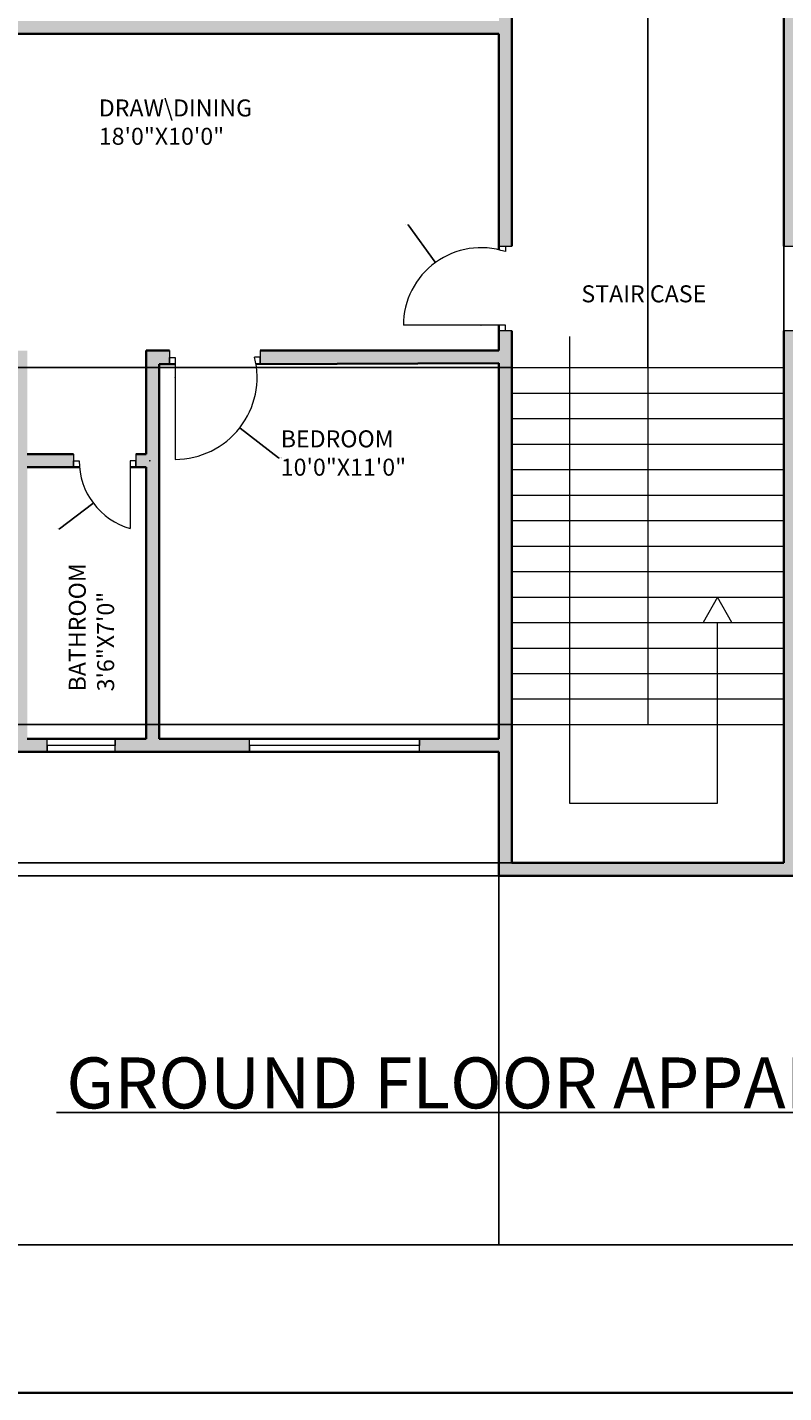
# Model space of a CAD drawing. Units: inches. Extents: x 2314 to 3223, y 1382 to 2735.
# Tile 2 of 14: x 2551 to 2818, y 1382 to 1864. Entities that reach past the tile are written whole.
import ezdxf

# ---------------------------------------------------------------- set-up
doc = ezdxf.new("R2010")
doc.units = ezdxf.units.IN
for name, color, linetype, lineweight in [('A-ANNO-DIMS', 2, 'Continuous', 18), ('A-ANNO-TEXT', 7, 'Continuous', 25), ('A-ANNO-TTLB', 7, 'Continuous', 35), ('A-AREA-IDEN', 7, 'Continuous', 18), ('A-DOOR', 3, 'Continuous', 18), ('A-FLOR-STRS', 7, 'Continuous', 18), ('A-GLAZ', 4, 'Continuous', 18), ('A-WALL', 7, 'Continuous', 35)]:
    doc.layers.add(name, color=color, linetype=linetype, lineweight=lineweight)
doc.layers.add('A-WALL-PATT', color=251, linetype='Continuous', lineweight=13, true_color=0x636466)
doc.styles.get("Standard").update_dxf_attribs({"font": 'arial.ttf'})
doc.dimstyles.get("Standard").update_dxf_attribs({"dimtxt": 0.18, "dimasz": 0.18, "dimexe": 0.18, "dimexo": 0.0625, "dimgap": 0.09, "dimtad": 0, "dimtih": 1, "dimtoh": 1, "dimdec": 4, "dimzin": 0, "dimdsep": 46, "dimtxsty": 'Standard', "dimcen": 0.09, "dimadec": 0, "dimazin": 0, "dimtfac": 1, "dimtdec": 4, "dimtofl": 0, "dimtmove": 0, "dimatfit": 3, "dimfxl": 1, "dimtolj": 1, "dimtzin": 0, "dimarcsym": 0})

# ---------------------------------------------------------------- blocks, each defined once
blk = doc.blocks.new('WIN-PLAN-24')
for p, q in [((0, 24), (4.5, 24)), ((4.5, 24), (2.25, 24)), ((2.25, 24), (2.25, 0)), ((2.25, 0), (0, 0)), ((0, 0), (4.5, 0))]:
    blk.add_line(p, q)
blk = doc.blocks.new('WIN-PLAN-60')
for p, q in [((0, 4.5), (0, 0)), ((0, 0), (0, 2.25)), ((0, 2.25), (60, 2.25)), ((60, 2.25), (60, 4.5)), ((60, 4.5), (60, 0))]:
    blk.add_line(p, q)
blk = doc.blocks.new('*D29')
at = {"layer": 'A-ANNO-DIMS', "color": 0, "lineweight": -2, "transparency": 16777216}
for p, q in [((2410.39, 1608.32), (2410.39, 1434.13)), ((3125.89, 1608.32), (3125.89, 1434.13)), ((2410.57, 1434.31), (2767.75, 1434.31)), ((3125.71, 1434.31), (2768.54, 1434.31))]:
    blk.add_line(p, q, dxfattribs=at)
at = {"layer": 'A-ANNO-DIMS', "color": 0, "transparency": 16777216}
for points in [[(2410.57, 1434.34), (2410.57, 1434.28), (2410.39, 1434.31)], [(3125.71, 1434.34), (3125.71, 1434.28), (3125.89, 1434.31)]]:
    blk.add_solid(points, dxfattribs=at)
at = {"layer": 'Defpoints', "color": 0, "transparency": 16777216}
for p in [(2410.39, 1608.38), (3125.89, 1608.38), (3125.89, 1434.31)]:
    blk.add_point(p, dxfattribs=at)
at = {"layer": 'A-ANNO-DIMS', "color": 0, "transparency": 16777216, "insert": (2768.14, 1434.31), "char_height": 0.18, "attachment_point": 5}
blk.add_mtext('\\A1;715.5', dxfattribs=at)
blk = doc.blocks.new('*D31')
at = {"layer": 'A-ANNO-DIMS', "color": 0, "lineweight": -2, "transparency": 16777216}
for p, q in [((2410.33, 1608.38), (2363.51, 1608.38)), ((2363.69, 1608.2), (2363.69, 1586.68)), ((2363.69, 1564.8), (2363.69, 1586.32)), ((2717.83, 1564.62), (2363.51, 1564.62))]:
    blk.add_line(p, q, dxfattribs=at)
at = {"layer": 'A-ANNO-DIMS', "color": 0, "transparency": 16777216}
for points in [[(2363.66, 1608.2), (2363.72, 1608.2), (2363.69, 1608.38)], [(2363.66, 1564.8), (2363.72, 1564.8), (2363.69, 1564.62)]]:
    blk.add_solid(points, dxfattribs=at)
at = {"layer": 'Defpoints', "color": 0, "transparency": 16777216}
for p in [(2363.69, 1608.38), (2410.39, 1608.38), (2717.89, 1564.62)]:
    blk.add_point(p, dxfattribs=at)
at = {"layer": 'A-ANNO-DIMS', "color": 0, "transparency": 16777216, "insert": (2363.69, 1586.5), "char_height": 0.18, "attachment_point": 5}
blk.add_mtext('\\A1;43.76', dxfattribs=at)
blk = doc.blocks.new('*D35')
at = {"layer": 'A-ANNO-DIMS', "color": 0, "lineweight": -2, "transparency": 16777216}
for p, q in [((2722.33, 1744), (2363.51, 1744)), ((2363.69, 1743.82), (2363.69, 1681.18)), ((2363.69, 1618.18), (2363.69, 1680.82)), ((2722.33, 1618), (2363.51, 1618))]:
    blk.add_line(p, q, dxfattribs=at)
at = {"layer": 'A-ANNO-DIMS', "color": 0, "transparency": 16777216}
for points in [[(2363.66, 1743.82), (2363.72, 1743.82), (2363.69, 1744)], [(2363.66, 1618.18), (2363.72, 1618.18), (2363.69, 1618)]]:
    blk.add_solid(points, dxfattribs=at)
at = {"layer": 'Defpoints', "color": 0, "transparency": 16777216}
for p in [(2363.69, 1744), (2722.39, 1744), (2722.39, 1618)]:
    blk.add_point(p, dxfattribs=at)
at = {"layer": 'A-ANNO-DIMS', "color": 0, "transparency": 16777216, "insert": (2363.69, 1681), "char_height": 0.18, "attachment_point": 5}
blk.add_mtext('\\A1;126', dxfattribs=at)
blk = doc.blocks.new('*D36')
at = {"layer": 'A-ANNO-DIMS', "color": 0, "lineweight": -2, "transparency": 16777216}
for p, q in [((2722.33, 1618), (2363.51, 1618)), ((2363.69, 1617.82), (2363.69, 1593.74)), ((2363.69, 1569.3), (2363.69, 1593.38)), ((2722.33, 1569.12), (2363.51, 1569.12))]:
    blk.add_line(p, q, dxfattribs=at)
at = {"layer": 'A-ANNO-DIMS', "color": 0, "transparency": 16777216}
for points in [[(2363.66, 1617.82), (2363.72, 1617.82), (2363.69, 1618)], [(2363.66, 1569.3), (2363.72, 1569.3), (2363.69, 1569.12)]]:
    blk.add_solid(points, dxfattribs=at)
at = {"layer": 'Defpoints', "color": 0, "transparency": 16777216}
for p in [(2363.69, 1618), (2722.39, 1618), (2722.39, 1569.12)]:
    blk.add_point(p, dxfattribs=at)
at = {"layer": 'A-ANNO-DIMS', "color": 0, "transparency": 16777216, "insert": (2363.69, 1593.56), "char_height": 0.18, "attachment_point": 5}
blk.add_mtext('\\A1;48.88', dxfattribs=at)
blk = doc.blocks.new('*D37')
at = {"layer": 'A-ANNO-DIMS', "color": 0, "lineweight": -2, "transparency": 16777216}
for p, q in [((2717.89, 1564.56), (2717.89, 1434.13)), ((2822.89, 1564.56), (2822.89, 1434.13)), ((2718.07, 1434.31), (2770.11, 1434.31)), ((2822.71, 1434.31), (2770.67, 1434.31))]:
    blk.add_line(p, q, dxfattribs=at)
at = {"layer": 'A-ANNO-DIMS', "color": 0, "transparency": 16777216}
for points in [[(2718.07, 1434.34), (2718.07, 1434.28), (2717.89, 1434.31)], [(2822.71, 1434.34), (2822.71, 1434.28), (2822.89, 1434.31)]]:
    blk.add_solid(points, dxfattribs=at)
at = {"layer": 'Defpoints', "color": 0, "transparency": 16777216}
for p in [(2717.89, 1564.62), (2822.89, 1564.62), (2822.89, 1434.31)]:
    blk.add_point(p, dxfattribs=at)
at = {"layer": 'A-ANNO-DIMS', "color": 0, "transparency": 16777216, "insert": (2770.39, 1434.31), "char_height": 0.18, "attachment_point": 5}
blk.add_mtext('\\A1;105', dxfattribs=at)
blk = doc.blocks.new('*D39')
at = {"layer": 'A-ANNO-DIMS', "color": 0, "lineweight": -2, "transparency": 16777216}
for p, q in [((2770.39, 1744.06), (2770.39, 2428.66)), ((2770.57, 2428.48), (2794.17, 2428.48)), ((2818.21, 2428.48), (2794.62, 2428.48)), ((2818.39, 1744.06), (2818.39, 2428.66))]:
    blk.add_line(p, q, dxfattribs=at)
at = {"layer": 'A-ANNO-DIMS', "color": 0, "transparency": 16777216}
for points in [[(2770.57, 2428.51), (2770.57, 2428.45), (2770.39, 2428.48)], [(2818.21, 2428.51), (2818.21, 2428.45), (2818.39, 2428.48)]]:
    blk.add_solid(points, dxfattribs=at)
at = {"layer": 'Defpoints', "color": 0, "transparency": 16777216}
for p in [(2818.39, 2428.48), (2770.39, 1744), (2818.39, 1744)]:
    blk.add_point(p, dxfattribs=at)
at = {"layer": 'A-ANNO-DIMS', "color": 0, "transparency": 16777216, "insert": (2794.39, 2428.48), "char_height": 0.18, "attachment_point": 5}
blk.add_mtext('\\A1;48', dxfattribs=at)
blk = doc.blocks.new('*D71')
at = {"layer": 'A-ANNO-DIMS', "color": 0, "lineweight": -2, "transparency": 16777216}
for p, q in [((2603.49, 1740.53), (2603.67, 1740.53)), ((2603.58, 1740.44), (2603.58, 1740.62)), ((2640.12, 1712.09), (2626.56, 1722.65)), ((2640.3, 1712.09), (2640.12, 1712.09))]:
    blk.add_line(p, q, dxfattribs=at)
at = {"layer": 'A-ANNO-DIMS', "color": 0, "transparency": 16777216}
blk.add_solid([(2626.58, 1722.67), (2626.54, 1722.62), (2626.42, 1722.76)], dxfattribs=at)
at = {"layer": 'Defpoints', "color": 0, "transparency": 16777216}
for p in [(2603.58, 1740.53), (2626.42, 1722.76)]:
    blk.add_point(p, dxfattribs=at)
at = {"layer": 'A-ANNO-DIMS', "color": 0, "transparency": 16777216, "insert": (2640.78, 1712.09), "char_height": 0.18, "attachment_point": 5}
blk.add_mtext('\\A1;R28.94', dxfattribs=at)
blk = doc.blocks.new('*D76')
at = {"layer": 'A-ANNO-DIMS', "color": 0, "lineweight": -2, "transparency": 16777216}
for p, q in [((2685.69, 1794.45), (2685.87, 1794.45)), ((2685.87, 1794.45), (2695.39, 1781.27)), ((2711.45, 1758.92), (2711.63, 1758.92)), ((2711.54, 1758.83), (2711.54, 1759.01))]:
    blk.add_line(p, q, dxfattribs=at)
at = {"layer": 'A-ANNO-DIMS', "color": 0, "transparency": 16777216}
blk.add_solid([(2695.41, 1781.29), (2695.37, 1781.25), (2695.5, 1781.12)], dxfattribs=at)
at = {"layer": 'Defpoints', "color": 0, "transparency": 16777216}
for p in [(2695.5, 1781.12), (2711.54, 1758.92)]:
    blk.add_point(p, dxfattribs=at)
at = {"layer": 'A-ANNO-DIMS', "color": 0, "transparency": 16777216, "insert": (2685.14, 1794.45), "char_height": 0.18, "attachment_point": 5}
blk.add_mtext('\\A1;R27.393', dxfattribs=at)
blk = doc.blocks.new('*D81')
at = {"layer": 'A-ANNO-DIMS', "color": 0, "lineweight": -2, "transparency": 16777216}
for p, q in [((2594.56, 1711.13), (2594.74, 1711.13)), ((2594.65, 1711.04), (2594.65, 1711.22)), ((2562.74, 1687.09), (2574.56, 1696)), ((2562.56, 1687.09), (2562.74, 1687.09))]:
    blk.add_line(p, q, dxfattribs=at)
at = {"layer": 'A-ANNO-DIMS', "color": 0, "transparency": 16777216}
blk.add_solid([(2574.54, 1696.02), (2574.58, 1695.98), (2574.7, 1696.11)], dxfattribs=at)
at = {"layer": 'Defpoints', "color": 0, "transparency": 16777216}
for p in [(2594.65, 1711.13), (2574.7, 1696.11)]:
    blk.add_point(p, dxfattribs=at)
at = {"layer": 'A-ANNO-DIMS', "color": 0, "transparency": 16777216, "insert": (2562.08, 1687.09), "char_height": 0.18, "attachment_point": 5}
blk.add_mtext('\\A1;R24.97', dxfattribs=at)

msp = doc.modelspace()

# ---------------------------------------------------------------- hatches: boundary and pattern name
at = {"layer": 'A-WALL-PATT'}
h = msp.add_hatch(color=256, dxfattribs=at)
h.dxf.hatch_style = 1
h.paths.add_polyline_path([(2443.3302, 2379.5332), (2443.3302, 2381.7832), (2410.3927, 2381.7832), (2410.3927, 2336.7008), (2414.8927, 2336.7008), (2414.8927, 2377.2832), (2443.3302, 2377.2832)])
h.paths.add_polyline_path([(2561.3645, 2379.5332), (2561.3645, 2381.7832), (2503.3302, 2381.7832), (2503.3302, 2377.2832), (2546.8927, 2377.2832), (2546.8927, 2245.2832), (2541.8787, 2245.2832), (2541.8787, 2240.7832), (2551.3927, 2240.7832), (2551.3927, 2377.2832), (2561.3645, 2377.2832)])
h.paths.add_polyline_path([(2656.0607, 2381.7832), (2597.3645, 2381.7832), (2597.3645, 2377.2832), (2617.3927, 2377.2832), (2617.3927, 2257.2832), (2584.2532, 2257.2832), (2584.2532, 2252.7832), (2625.8528, 2252.7832), (2625.8528, 2255.0332), (2625.8528, 2257.2832), (2621.8927, 2257.2832), (2621.8927, 2377.2832), (2656.0607, 2377.2832), (2656.0607, 2379.5332)])
h.paths.add_polyline_path([(2807.3418, 2381.7832), (2716.0607, 2381.7832), (2716.0607, 2377.2832), (2765.8927, 2377.2832), (2765.8927, 2257.2832), (2661.6935, 2257.2832), (2661.6935, 2252.7832), (2765.8927, 2252.7832), (2765.8927, 2146.2832), (2760.9259, 2146.2832), (2760.9259, 2141.8832), (2775.7119, 2141.8832), (2775.7119, 2146.2832), (2770.3927, 2146.2832), (2770.3927, 2252.7832), (2877.684, 2252.7832), (2877.684, 2255.0332), (2877.684, 2257.2832), (2770.3927, 2257.2832), (2770.3927, 2377.2832), (2807.3418, 2377.2832), (2807.3418, 2379.5332)])
h.paths.add_polyline_path([(2937.2118, 2381.7832), (2867.3418, 2381.7832), (2867.3418, 2377.2832), (2914.3927, 2377.2832), (2914.3927, 2257.2832), (2908.4124, 2257.2832), (2908.4124, 2252.7832), (2960.6432, 2252.7832), (2960.6432, 2255.0332), (2960.6432, 2257.2832), (2918.8927, 2257.2832), (2918.8927, 2377.2832), (2937.2118, 2377.2832)])
h.paths.add_polyline_path([(3022.1601, 2381.7832), (2973.2118, 2381.7832), (2973.2118, 2379.5332), (2973.2118, 2377.2832), (2984.8927, 2377.2832), (2984.8927, 2257.2832), (2980.0601, 2257.2832), (2980.0601, 2252.7832), (2984.8927, 2252.7832), (2984.8927, 2240.7832), (2995.668, 2240.7832), (2995.668, 2243.0332), (2995.668, 2245.2832), (2989.3927, 2245.2832), (2989.3927, 2377.2832), (3022.1601, 2377.2832), (3022.1601, 2379.5332)])
h.paths.add_polyline_path([(3125.8927, 2381.7832), (3082.1601, 2381.7832), (3082.1601, 2377.2832), (3121.3927, 2377.2832), (3121.3927, 2334.7388), (3125.8927, 2334.7388)])
h.paths.add_polyline_path([(3125.8927, 2274.7388), (3121.3927, 2274.7388), (3121.3927, 2245.2832), (3066.4832, 2245.2832), (3066.4832, 2240.7832), (3121.3927, 2240.7832), (3121.3927, 2232.1868), (3125.8927, 2232.1868)])
h.paths.add_polyline_path([(3125.8927, 2208.1868), (3121.3927, 2208.1868), (3121.3927, 2198.7832), (3037.3927, 2198.7832), (3037.3927, 2240.7832), (3041.2694, 2240.7832), (3041.2694, 2243.0332), (3041.2694, 2245.2832), (3026.8205, 2245.2832), (3026.8205, 2240.7832), (3032.8927, 2240.7832), (3032.8927, 2190.4022), (3037.3927, 2190.4022), (3037.3927, 2194.2832), (3121.3927, 2194.2832), (3121.3927, 2182.1835), (3125.8927, 2182.1835)])
h.paths.add_polyline_path([(3125.8927, 2158.1835), (3121.3927, 2158.1835), (3121.3927, 2146.2832), (3037.3927, 2146.2832), (3037.3927, 2169.3726), (3035.1427, 2169.3726), (3032.8927, 2169.3726), (3032.8927, 2146.2832), (2812.7301, 2146.2832), (2812.7301, 2144.0832), (2812.7301, 2141.8832), (2818.3927, 2141.8832), (2818.3927, 1970.1316), (2822.8927, 1970.1316), (2822.8927, 1978.8832), (2903.9846, 1978.8832), (2903.9846, 1981.1332), (2903.9846, 1983.3832), (2822.8927, 1983.3832), (2822.8927, 2115.3832), (2851.7162, 2115.3832), (2851.7162, 2117.6332), (2851.7162, 2119.8832), (2822.8927, 2119.8832), (2822.8927, 2141.8832), (3125.8927, 2141.8832)])
h.paths.add_polyline_path([(3125.8927, 2119.8832), (3081.193, 2119.8832), (3081.193, 2115.3832), (3121.3927, 2115.3832), (3121.3927, 2071.8188), (3125.8927, 2071.8188)], flags=17)
h.paths.add_polyline_path([(2989.3927, 2115.3832), (3021.193, 2115.3832), (3021.193, 2117.6332), (3021.193, 2119.8832), (2979.123, 2119.8832), (2979.123, 2115.3832), (2984.8927, 2115.3832), (2984.8927, 2019.3832), (2981.9225, 2019.3832), (2981.9225, 2014.8832), (2984.8927, 2014.8832), (2984.8927, 1983.3832), (2984.8927, 1978.8832), (2989.3927, 1978.8832), (2989.3927, 1983.3832)], flags=17)
h.paths.add_polyline_path([(2947.3927, 2115.3832), (2955.123, 2115.3832), (2955.123, 2117.6332), (2955.123, 2119.8832), (2911.7162, 2119.8832), (2911.7162, 2115.3832), (2942.8927, 2115.3832), (2942.8927, 1983.3832), (2936.7017, 1983.3832), (2936.7017, 1978.8832), (2947.3927, 1978.8832), (2947.3927, 1983.3832), (2947.3927, 2014.8832), (2960.7167, 2014.8832), (2960.7167, 2017.1332), (2960.7167, 2019.3832), (2947.3927, 2019.3832)], flags=17)
h.paths.add_polyline_path([(3037.3927, 1978.8832), (3041.8276, 1978.8832), (3041.8276, 1981.1332), (3041.8276, 1983.3832), (3025.477, 1983.3832), (3025.477, 1978.8832), (3032.8927, 1978.8832), (3032.8927, 1927.1259), (3035.1427, 1927.1259), (3037.3927, 1927.1259)])
h.paths.add_polyline_path([(3125.8927, 2011.8188), (3123.6427, 2011.8188), (3121.3927, 2011.8188), (3121.3927, 1983.3832), (3065, 1983.3832), (3065, 1978.8832), (3121.3927, 1978.8832), (3121.3927, 1970.5932), (3125.8927, 1970.5932)], flags=17)
h.paths.add_polyline_path([(2994.2341, 1983.3832), (2989.3927, 1983.3832), (2989.3927, 1978.8832), (2994.2341, 1978.8832), (2994.2341, 1981.1332)], flags=16)
h.paths.add_polyline_path([(3125.8927, 1946.5932), (3121.3927, 1946.5932), (3121.3927, 1936.8832), (3037.3927, 1936.8832), (3037.3927, 1932.3832), (3121.3927, 1932.3832), (3121.3927, 1919.825), (3125.8927, 1919.825)])
h.paths.add_polyline_path([(3125.8927, 1883.825), (3121.3927, 1883.825), (3121.3927, 1866.3832), (3037.3927, 1866.3832), (3037.3927, 1899.0954), (3035.1427, 1899.0954), (3032.8927, 1899.0954), (3032.8927, 1866.3832), (2822.8927, 1866.3832), (2822.8927, 1938.7212), (2820.6427, 1938.7212), (2818.3927, 1938.7212), (2818.3927, 1786.9239), (2822.8927, 1786.9239), (2822.8927, 1861.8832), (3032.8927, 1861.8832), (3032.8927, 1825.1023), (3037.3927, 1825.1023), (3037.3927, 1861.8832), (3121.3927, 1861.8832), (3121.3927, 1844.6765), (3125.8927, 1844.6765)])
h.paths.add_polyline_path([(3125.8927, 1808.6765), (3121.3927, 1808.6765), (3121.3927, 1795.8832), (3037.3927, 1795.8832), (3037.3927, 1799.4755), (3032.8927, 1799.4755), (3032.8927, 1749.3832), (3026.5034, 1749.3832), (3026.5034, 1744.8832), (3032.8927, 1744.8832), (3034.9255, 1744.8832), (3043.1326, 1744.8832), (3043.1326, 1747.1332), (3043.1326, 1749.3832), (3037.3927, 1749.3832), (3037.3927, 1791.3832), (3121.3927, 1791.3832), (3121.3927, 1783.3103), (3125.8927, 1783.3103)])
h.paths.add_polyline_path([(3125.8927, 1759.3103), (3121.3927, 1759.3103), (3121.3927, 1749.3832), (3065.1845, 1749.3832), (3065.1845, 1744.8832), (3121.3927, 1744.8832), (3121.3927, 1709.3573), (3125.8927, 1709.3573)])
h.paths.add_polyline_path([(3125.8927, 1649.3573), (3121.3927, 1649.3573), (3121.3927, 1612.8832), (3095.116, 1612.8832), (3095.116, 1608.3832), (3125.8927, 1608.3832)])
h.paths.add_polyline_path([(3035.116, 1612.8832), (2993.8927, 1612.8832), (2993.8927, 1744.8832), (2998.7409, 1744.8832), (2998.7409, 1749.3832), (2989.3927, 1749.3832), (2989.3927, 1744.8832), (2989.3927, 1701.3832), (2972.8226, 1701.3832), (2972.8226, 1696.8832), (2989.3927, 1696.8832), (2989.3927, 1612.8832), (2978.2225, 1612.8832), (2978.2225, 1608.3832), (3035.116, 1608.3832), (3035.116, 1610.6332)])
h.paths.add_polyline_path([(2947.3927, 1696.8832), (2950.7566, 1696.8832), (2950.7566, 1699.1332), (2950.7566, 1701.3832), (2947.3927, 1701.3832), (2947.3927, 1744.8832), (2947.3927, 1749.3832), (2937.649, 1749.3832), (2937.649, 1744.8832), (2942.8927, 1744.8832), (2942.8927, 1612.8832), (2907.783, 1612.8832), (2907.783, 1608.3832), (2954.2225, 1608.3832), (2954.2225, 1610.6332), (2954.2225, 1612.8832), (2947.3927, 1612.8832)])
h.paths.add_polyline_path([(2822.8927, 1744.8832), (2905.3491, 1744.8832), (2905.3491, 1747.1332), (2905.3491, 1749.3832), (2822.8927, 1749.3832), (2822.8927, 1756.9185), (2818.3927, 1756.9185), (2818.3927, 1612.8832), (2818.3927, 1569.1205), (2722.3927, 1569.1205), (2722.3927, 1612.8832), (2722.3927, 1756.9185), (2717.8927, 1756.9185), (2717.8927, 1750.0143), (2633.6297, 1750.0143), (2633.6437, 1745.2665), (2717.8927, 1745.5143), (2717.8927, 1612.8832), (2689.8467, 1612.8832), (2689.8467, 1608.3832), (2717.8927, 1608.3832), (2717.8927, 1564.6205), (2722.3927, 1564.6205), (2822.8927, 1564.6205), (2822.8927, 1569.1205), (2822.8927, 1608.3832), (2847.783, 1608.3832), (2847.783, 1610.6332), (2847.783, 1612.8832), (2822.8927, 1612.8832)])
h.paths.add_polyline_path([(2629.8467, 1612.8832), (2597.8927, 1612.8832), (2597.8927, 1744.8832), (2597.8927, 1745.1613), (2601.5887, 1745.1721), (2601.5816, 1747.5932), (2601.5745, 1750.0143), (2593.3927, 1750.0143), (2593.3927, 1744.8832), (2593.3927, 1713.3832), (2589.7588, 1713.3832), (2589.7588, 1708.8832), (2593.3927, 1708.8832), (2593.3927, 1612.8832), (2582.3793, 1612.8832), (2582.3793, 1608.3832), (2629.8467, 1608.3832), (2629.8467, 1610.6332)])
h.paths.add_polyline_path([(2551.3927, 1708.8832), (2567.6776, 1708.8832), (2567.6776, 1711.1332), (2567.6776, 1713.3832), (2551.3927, 1713.3832), (2551.3927, 1744.8832), (2551.3927, 1750.0143), (2543.5657, 1750.0143), (2543.5657, 1747.5079), (2543.5657, 1745.0014), (2546.8927, 1745.0112), (2546.8927, 1744.8832), (2546.8927, 1612.8832), (2502.9339, 1612.8832), (2502.9339, 1608.3832), (2558.3793, 1608.3832), (2558.3793, 1610.6332), (2558.3793, 1612.8832), (2551.3927, 1612.8832)])
h.paths.add_polyline_path([(2414.8927, 1656.2547), (2410.3927, 1656.2547), (2410.3927, 1608.3832), (2442.9339, 1608.3832), (2442.9339, 1610.6332), (2442.9339, 1612.8832), (2414.8927, 1612.8832)])
h.paths.add_polyline_path([(2414.8927, 1744.8832), (2468.8906, 1744.8832), (2468.8906, 1747.1332), (2468.8906, 1749.3832), (2414.8927, 1749.3832), (2414.8927, 1757.7622), (2410.3927, 1757.7622), (2410.3927, 1716.2547), (2414.8927, 1716.2547)])
h.paths.add_polyline_path([(2414.8927, 1791.3832), (2498.8927, 1791.3832), (2498.8927, 1749.3832), (2492.9799, 1749.3832), (2492.9799, 1744.8832), (2498.8927, 1744.8832), (2503.3927, 1744.8832), (2508.0135, 1744.8968), (2508.0059, 1747.4556), (2507.9984, 1750.0143), (2503.3927, 1750.0143), (2503.3927, 1802.6362), (2501.1427, 1802.6362), (2498.8927, 1802.6362), (2498.8927, 1795.8832), (2414.8927, 1795.8832), (2414.8927, 1808.0943), (2410.3927, 1808.0943), (2410.3927, 1781.7622), (2414.8927, 1781.7622)])
h.paths.add_polyline_path([(2722.3927, 1937.589), (2720.1427, 1937.589), (2717.8927, 1937.589), (2717.8927, 1866.3832), (2503.3927, 1866.3832), (2503.3927, 1896.3484), (2498.8927, 1896.3484), (2498.8927, 1866.3832), (2414.8927, 1866.3832), (2414.8927, 1882.1496), (2410.3927, 1882.1496), (2410.3927, 1844.0943), (2414.8927, 1844.0943), (2414.8927, 1861.8832), (2498.8927, 1861.8832), (2498.8927, 1831.4783), (2501.1427, 1831.4783), (2503.3927, 1831.4783), (2503.3927, 1861.8832), (2717.8927, 1861.8832), (2717.8927, 1786.9239), (2722.3927, 1786.9239)])
h.paths.add_polyline_path([(2414.8927, 1932.3832), (2498.8927, 1932.3832), (2498.8927, 1924.7883), (2503.3927, 1924.7883), (2503.3927, 1978.8832), (2505.8599, 1978.8832), (2505.8599, 1981.1332), (2505.8599, 1983.3832), (2493.3697, 1983.3832), (2493.3697, 1978.8832), (2498.8927, 1978.8832), (2498.8927, 1936.8832), (2414.8927, 1936.8832), (2414.8927, 1943.2834), (2410.3927, 1943.2834), (2410.3927, 1918.1496), (2414.8927, 1918.1496)])
h.paths.add_polyline_path([(2414.8927, 2020.3133), (2412.6427, 2020.3133), (2410.3927, 2020.3133), (2410.3927, 1967.2834), (2414.8927, 1967.2834), (2414.8927, 1978.8832), (2468.8513, 1978.8832), (2468.8513, 1981.1332), (2468.8513, 1983.3832), (2414.8927, 1983.3832)])
h.paths.add_polyline_path([(2414.8927, 2115.3832), (2453.004, 2115.3832), (2453.004, 2117.6332), (2453.004, 2119.8832), (2410.3927, 2119.8832), (2410.3927, 2080.3133), (2414.8927, 2080.3133)], flags=17)
h.paths.add_polyline_path([(2559.0969, 2117.6332), (2559.0969, 2119.8832), (2513.004, 2119.8832), (2513.004, 2115.3832), (2546.8927, 2115.3832), (2546.8927, 1983.3832), (2542.7531, 1983.3832), (2542.7531, 1978.8832), (2551.3927, 1978.8832), (2551.3927, 2014.8832), (2570.3098, 2014.8832), (2570.3098, 2017.1332), (2570.3098, 2019.3832), (2551.3927, 2019.3832), (2551.3927, 2115.3832), (2559.0969, 2115.3832)], flags=17)
h.paths.add_polyline_path([(2628.5073, 2117.6332), (2628.5073, 2119.8832), (2583.0969, 2119.8832), (2583.0969, 2115.3832), (2593.3927, 2115.3832), (2593.3927, 2019.3832), (2590.2108, 2019.3832), (2590.2108, 2014.8832), (2593.3927, 2014.8832), (2593.3927, 1978.8832), (2601.5907, 1978.8832), (2601.5907, 1981.1332), (2601.5907, 1983.3832), (2597.8927, 1983.3832), (2597.8927, 2115.3832), (2628.5073, 2115.3832)], flags=17)
h.paths.add_polyline_path([(2722.3927, 2141.8832), (2726.9871, 2141.8832), (2726.9871, 2144.2705), (2726.9871, 2146.2832), (2503.3927, 2146.2832), (2503.3927, 2168.2161), (2501.1427, 2168.2161), (2498.8927, 2168.2161), (2498.8927, 2146.2832), (2414.8927, 2146.2832), (2414.8927, 2156.5041), (2410.3927, 2156.5041), (2410.3927, 2141.8832), (2717.8927, 2141.8832), (2717.8927, 2119.8832), (2688.5073, 2119.8832), (2688.5073, 2115.3832), (2717.8927, 2115.3832), (2717.8927, 1983.3832), (2633.2454, 1983.3832), (2633.2454, 1978.8832), (2717.8927, 1978.8832), (2717.8927, 1970.1316), (2720.1427, 1970.1316), (2722.3927, 1970.1316)])
h.paths.add_polyline_path([(2557.3704, 1462.9278), (2940.0934, 1462.9278), (2940.0934, 1512.3848), (2557.3704, 1512.3848)], flags=9)
h.paths.add_polyline_path([(2846.2527, 1703.1384), (2892.8612, 1703.1384), (2892.8612, 1725.5272), (2846.2527, 1725.5272)], flags=25)
h.paths.add_polyline_path([(2885.6102, 1812.1147), (2946.1505, 1812.1147), (2946.1505, 1834.5035), (2885.6102, 1834.5035)], flags=25)
h.paths.add_polyline_path([(2885.6102, 1884.183), (2946.1505, 1884.183), (2946.1505, 1906.5718), (2885.6102, 1906.5718)], flags=25)
h.paths.add_polyline_path([(3066.365, 1705.5431), (3112.9735, 1705.5431), (3112.9735, 1727.9319), (3066.365, 1727.9319)], flags=9)
h.paths.add_polyline_path([(3061.8255, 1887.7513), (3101.6154, 1887.7513), (3101.6154, 1910.1401), (3061.8255, 1910.1401)], flags=25)
h.paths.add_polyline_path([(3063.3679, 1816.2121), (3103.1578, 1816.2121), (3103.1578, 1838.6009), (3063.3679, 1838.6009)], flags=25)
h.paths.add_polyline_path([(3053.3743, 1768.416), (3107.1329, 1768.416), (3107.1329, 1790.8048), (3053.3743, 1790.8048)], flags=25)
h.paths.add_polyline_path([(3061.6068, 1943.822), (3115.3653, 1943.822), (3115.3653, 1966.2109), (3061.6068, 1966.2109)], flags=9)
h.paths.add_polyline_path([(2745.0978, 1763.6604), (2797.9354, 1763.6604), (2797.9354, 1776.0247), (2745.0978, 1776.0247)], flags=9)
h.paths.add_polyline_path([(2574.2135, 1819.2586), (2634.7538, 1819.2586), (2634.7538, 1841.6474), (2574.2135, 1841.6474)], flags=25)
h.paths.add_polyline_path([(2574.2135, 1891.3269), (2634.7538, 1891.3269), (2634.7538, 1913.7157), (2574.2135, 1913.7157)], flags=25)
h.paths.add_polyline_path([(2638.4466, 1702.43), (2685.0551, 1702.43), (2685.0551, 1724.8188), (2638.4466, 1724.8188)], flags=25)
h.paths.add_polyline_path([(2435.9715, 1697.1215), (2482.5799, 1697.1215), (2482.5799, 1719.5103), (2435.9715, 1719.5103)], flags=9)
h.paths.add_polyline_path([(2431.2046, 1893.7833), (2470.9945, 1893.7833), (2470.9945, 1916.1721), (2431.2046, 1916.1721)], flags=25)
h.paths.add_polyline_path([(2439.8144, 1817.2116), (2479.6043, 1817.2116), (2479.6043, 1839.6004), (2439.8144, 1839.6004)], flags=25)
h.paths.add_polyline_path([(2441.2607, 1753.0942), (2495.0192, 1753.0942), (2495.0192, 1775.483), (2441.2607, 1775.483)], flags=25)
h.paths.add_polyline_path([(2421.216, 1945.3109), (2474.9746, 1945.3109), (2474.9746, 1967.6997), (2421.216, 1967.6997)], flags=25)
h.paths.add_polyline_path([(2585.4464, 1627.5703), (2585.4464, 1679), (2563.0576, 1679), (2563.0576, 1627.5703)], flags=9)
h.paths.add_polyline_path([(2978.3497, 1618.7039), (2978.3497, 1670.1337), (2955.9609, 1670.1337), (2955.9609, 1618.7039)], flags=9)
h.paths.add_polyline_path([(2975.9502, 2041.7828), (2975.9502, 2093.2125), (2953.5614, 2093.2125), (2953.5614, 2041.7828)], flags=25)
h.paths.add_polyline_path([(2835.6537, 1989.2068), (2882.2621, 1989.2068), (2882.2621, 2011.5956), (2835.6537, 2011.5956)], flags=25)
h.paths.add_polyline_path([(2649.3769, 1997.5659), (2695.9853, 1997.5659), (2695.9853, 2019.9547), (2649.3769, 2019.9547)], flags=25)
h.paths.add_polyline_path([(2579.9087, 2040.3429), (2579.9087, 2091.7726), (2557.5198, 2091.7726), (2557.5198, 2040.3429)], flags=25)
h.paths.add_polyline_path([(2783.2404, 1883.1956), (2783.2404, 2067.1369), (2764.694, 2067.1369), (2764.694, 1883.1956)], flags=9)
h.paths.add_polyline_path([(3055.8435, 1993.5571), (3102.4519, 1993.5571), (3102.4519, 2015.9459), (3055.8435, 2015.9459)], flags=25)
h.paths.add_polyline_path([(2423.6009, 1984.6082), (2470.2094, 1984.6082), (2470.2094, 2006.997), (2423.6009, 2006.997)], flags=25)
h.paths.add_polyline_path([(2973.4115, 2123.1668), (3013.1319, 2123.1668), (3013.1319, 2135.531), (2973.4115, 2135.531)], flags=25)
h.paths.add_polyline_path([(2534.3846, 2124.6231), (2574.105, 2124.6231), (2574.105, 2136.9874), (2534.3846, 2136.9874)], flags=25)
h.paths.add_polyline_path([(2829.1368, 2188.1931), (2889.411, 2188.1931), (2889.411, 2210.5819), (2829.1368, 2210.5819)], flags=9)
h.paths.add_polyline_path([(2633.2547, 2185.0437), (2693.5289, 2185.0437), (2693.5289, 2207.4325), (2633.2547, 2207.4325)], flags=9)
h.paths.add_polyline_path([(2445.1812, 2167.0395), (2496.611, 2167.0395), (2496.611, 2189.4284), (2445.1812, 2189.4284)], flags=9)
h.paths.add_polyline_path([(2429.1678, 2194.5482), (2480.5975, 2194.5482), (2480.5975, 2216.937), (2429.1678, 2216.937)], flags=9)
h.paths.add_polyline_path([(3060.1138, 2158.1056), (3111.5436, 2158.1056), (3111.5436, 2180.4944), (3060.1138, 2180.4944)], flags=9)
h.paths.add_polyline_path([(3055.6824, 2201.2631), (3107.1122, 2201.2631), (3107.1122, 2223.652), (3055.6824, 2223.652)], flags=25)
h.paths.add_polyline_path([(3044.3482, 2257.7345), (3090.9567, 2257.7345), (3090.9567, 2280.1233), (3044.3482, 2280.1233)], flags=9)
h.paths.add_polyline_path([(2942.5437, 2306.9625), (2982.3336, 2306.9625), (2982.3336, 2329.3513), (2942.5437, 2329.3513)], flags=9)
h.paths.add_polyline_path([(2799.5865, 2259.1663), (2846.195, 2259.1663), (2846.195, 2281.5551), (2799.5865, 2281.5551)], flags=25)
h.paths.add_polyline_path([(2670.4998, 2261.1493), (2717.1082, 2261.1493), (2717.1082, 2283.5381), (2670.4998, 2283.5381)], flags=25)
h.paths.add_polyline_path([(2553.0333, 2302.7735), (2592.8232, 2302.7735), (2592.8232, 2325.1624), (2553.0333, 2325.1624)], flags=9)
h.paths.add_polyline_path([(2432.0288, 2268.6489), (2478.6372, 2268.6489), (2478.6372, 2291.0377), (2432.0288, 2291.0377)], flags=9)
h = msp.add_hatch(color=256, dxfattribs=at)
h.dxf.hatch_style = 1
h.paths.add_polyline_path([(2503.3927, 2240.7832), (2507.7952, 2240.7832), (2507.7952, 2245.2832), (2496.4262, 2245.2832), (2496.4262, 2243.0332), (2496.4262, 2240.7832), (2498.8927, 2240.7832), (2498.8927, 2198.7832), (2414.8927, 2198.7832), (2414.8927, 2206.5718), (2410.3927, 2206.5718), (2410.3927, 2180.5041), (2412.6427, 2180.5041), (2414.8927, 2180.5041), (2414.8927, 2194.2832), (2498.8927, 2194.2832), (2498.8927, 2191.0069), (2503.3927, 2191.0069)])
h.paths.add_polyline_path([(2414.8927, 2276.7008), (2410.3927, 2276.7008), (2410.3927, 2230.5718), (2414.8927, 2230.5718), (2414.8927, 2240.7832), (2474.2564, 2240.7832), (2474.2564, 2243.0332), (2474.2564, 2245.2832), (2414.8927, 2245.2832)])
h.paths.add_polyline_path([(2557.3704, 1462.9278), (2940.0934, 1462.9278), (2940.0934, 1512.3848), (2557.3704, 1512.3848)], flags=9)
h.paths.add_polyline_path([(2846.2527, 1703.1384), (2892.8612, 1703.1384), (2892.8612, 1725.5272), (2846.2527, 1725.5272)], flags=9)
h.paths.add_polyline_path([(2885.6102, 1812.1147), (2946.1505, 1812.1147), (2946.1505, 1834.5035), (2885.6102, 1834.5035)], flags=9)
h.paths.add_polyline_path([(2885.6102, 1884.183), (2946.1505, 1884.183), (2946.1505, 1906.5718), (2885.6102, 1906.5718)], flags=9)
h.paths.add_polyline_path([(3066.365, 1705.5431), (3112.9735, 1705.5431), (3112.9735, 1727.9319), (3066.365, 1727.9319)], flags=9)
h.paths.add_polyline_path([(3061.8255, 1887.7513), (3101.6154, 1887.7513), (3101.6154, 1910.1401), (3061.8255, 1910.1401)], flags=9)
h.paths.add_polyline_path([(3063.3679, 1816.2121), (3103.1578, 1816.2121), (3103.1578, 1838.6009), (3063.3679, 1838.6009)], flags=9)
h.paths.add_polyline_path([(3053.3743, 1768.416), (3107.1329, 1768.416), (3107.1329, 1790.8048), (3053.3743, 1790.8048)], flags=9)
h.paths.add_polyline_path([(3061.6068, 1943.822), (3115.3653, 1943.822), (3115.3653, 1966.2109), (3061.6068, 1966.2109)], flags=9)
h.paths.add_polyline_path([(2745.0978, 1763.6604), (2797.9354, 1763.6604), (2797.9354, 1776.0247), (2745.0978, 1776.0247)], flags=9)
h.paths.add_polyline_path([(2574.2135, 1819.2586), (2634.7538, 1819.2586), (2634.7538, 1841.6474), (2574.2135, 1841.6474)], flags=9)
h.paths.add_polyline_path([(2574.2135, 1891.3269), (2634.7538, 1891.3269), (2634.7538, 1913.7157), (2574.2135, 1913.7157)], flags=9)
h.paths.add_polyline_path([(2638.4466, 1702.43), (2685.0551, 1702.43), (2685.0551, 1724.8188), (2638.4466, 1724.8188)], flags=9)
h.paths.add_polyline_path([(2435.9715, 1697.1215), (2482.5799, 1697.1215), (2482.5799, 1719.5103), (2435.9715, 1719.5103)], flags=9)
h.paths.add_polyline_path([(2431.2046, 1893.7833), (2470.9945, 1893.7833), (2470.9945, 1916.1721), (2431.2046, 1916.1721)], flags=9)
h.paths.add_polyline_path([(2439.8144, 1817.2116), (2479.6043, 1817.2116), (2479.6043, 1839.6004), (2439.8144, 1839.6004)], flags=9)
h.paths.add_polyline_path([(2441.2607, 1753.0942), (2495.0192, 1753.0942), (2495.0192, 1775.483), (2441.2607, 1775.483)], flags=9)
h.paths.add_polyline_path([(2421.216, 1945.3109), (2474.9746, 1945.3109), (2474.9746, 1967.6997), (2421.216, 1967.6997)], flags=9)
h.paths.add_polyline_path([(2585.4464, 1627.5703), (2585.4464, 1679), (2563.0576, 1679), (2563.0576, 1627.5703)], flags=9)
h.paths.add_polyline_path([(2978.3497, 1618.7039), (2978.3497, 1670.1337), (2955.9609, 1670.1337), (2955.9609, 1618.7039)], flags=9)
h.paths.add_polyline_path([(2975.9502, 2041.7828), (2975.9502, 2093.2125), (2953.5614, 2093.2125), (2953.5614, 2041.7828)], flags=9)
h.paths.add_polyline_path([(2835.6537, 1989.2068), (2882.2621, 1989.2068), (2882.2621, 2011.5956), (2835.6537, 2011.5956)], flags=9)
h.paths.add_polyline_path([(2649.3769, 1997.5659), (2695.9853, 1997.5659), (2695.9853, 2019.9547), (2649.3769, 2019.9547)], flags=9)
h.paths.add_polyline_path([(2579.9087, 2040.3429), (2579.9087, 2091.7726), (2557.5198, 2091.7726), (2557.5198, 2040.3429)], flags=9)
h.paths.add_polyline_path([(2783.2404, 1883.1956), (2783.2404, 2067.1369), (2764.694, 2067.1369), (2764.694, 1883.1956)], flags=9)
h.paths.add_polyline_path([(3055.8435, 1993.5571), (3102.4519, 1993.5571), (3102.4519, 2015.9459), (3055.8435, 2015.9459)], flags=9)
h.paths.add_polyline_path([(2423.6009, 1984.6082), (2470.2094, 1984.6082), (2470.2094, 2006.997), (2423.6009, 2006.997)], flags=9)
h.paths.add_polyline_path([(2973.4115, 2123.1668), (3013.1319, 2123.1668), (3013.1319, 2135.531), (2973.4115, 2135.531)], flags=9)
h.paths.add_polyline_path([(2534.3846, 2124.6231), (2574.105, 2124.6231), (2574.105, 2136.9874), (2534.3846, 2136.9874)], flags=9)
h.paths.add_polyline_path([(2829.1368, 2188.1931), (2889.411, 2188.1931), (2889.411, 2210.5819), (2829.1368, 2210.5819)], flags=9)
h.paths.add_polyline_path([(2633.2547, 2185.0437), (2693.5289, 2185.0437), (2693.5289, 2207.4325), (2633.2547, 2207.4325)], flags=9)
h.paths.add_polyline_path([(2445.1812, 2167.0395), (2496.611, 2167.0395), (2496.611, 2189.4284), (2445.1812, 2189.4284)], flags=9)
h.paths.add_polyline_path([(2429.1678, 2208.3022), (2480.5975, 2208.3022), (2480.5975, 2230.691), (2429.1678, 2230.691)], flags=25)
h.paths.add_polyline_path([(3060.1138, 2158.1056), (3111.5436, 2158.1056), (3111.5436, 2180.4944), (3060.1138, 2180.4944)], flags=9)
h.paths.add_polyline_path([(3055.6824, 2201.2631), (3107.1122, 2201.2631), (3107.1122, 2223.652), (3055.6824, 2223.652)], flags=9)
h.paths.add_polyline_path([(3044.3482, 2257.7345), (3090.9567, 2257.7345), (3090.9567, 2280.1233), (3044.3482, 2280.1233)], flags=9)
h.paths.add_polyline_path([(2942.5437, 2306.9625), (2982.3336, 2306.9625), (2982.3336, 2329.3513), (2942.5437, 2329.3513)], flags=9)
h.paths.add_polyline_path([(2799.5865, 2259.1663), (2846.195, 2259.1663), (2846.195, 2281.5551), (2799.5865, 2281.5551)], flags=9)
h.paths.add_polyline_path([(2670.4998, 2261.1493), (2717.1082, 2261.1493), (2717.1082, 2283.5381), (2670.4998, 2283.5381)], flags=9)
h.paths.add_polyline_path([(2553.0333, 2302.7735), (2592.8232, 2302.7735), (2592.8232, 2325.1624), (2553.0333, 2325.1624)], flags=9)
h.paths.add_polyline_path([(2432.0288, 2268.6489), (2478.6372, 2268.6489), (2478.6372, 2291.0377), (2432.0288, 2291.0377)], flags=9)

# ---------------------------------------------------------------- linework, layer by layer
at = {"layer": 'A-ANNO-TEXT'}
msp.add_line((2561.7354, 1481.0145), (3035.0613, 1481.0145), dxfattribs=at)
at = {"layer": 'A-ANNO-TTLB'}
msp.add_lwpolyline([(2314.008, 2735.417), (3222.6676, 2735.417), (3222.6676, 1382.0876), (2314.008, 1382.0876)], close=True, dxfattribs=at)
at = {"layer": 'A-DOOR'}
for p, q in [((2717.8927, 1786.9239), (2722.3927, 1786.9239)), ((2720.1427, 1786.9239), (2720.1427, 1784.9239)), ((2818.3927, 1786.9239), (2822.8927, 1786.9239)), ((2720.1427, 1758.9185), (2684.1427, 1758.9185)), ((2722.3927, 1756.9185), (2717.8927, 1756.9185)), ((2720.1427, 1756.9185), (2720.1427, 1758.9185)), ((2822.8927, 1756.9185), (2818.3927, 1756.9185)), ((2601.5745, 1750.0143), (2601.5887, 1745.1721)), ((2633.6297, 1750.0143), (2633.6437, 1745.2665)), ((2601.5887, 1745.1721), (2601.5816, 1747.5932)), ((2601.5816, 1747.5932), (2603.5816, 1747.5932)), ((2603.5816, 1747.5932), (2603.5816, 1711.5932)), ((2633.6367, 1747.6404), (2631.6367, 1747.6404)), ((2633.6437, 1745.2665), (2633.6367, 1747.6404)), ((2567.6776, 1713.3832), (2567.6776, 1708.8832)), ((2589.7588, 1713.3832), (2589.7588, 1708.8832)), ((2567.6776, 1708.8832), (2567.6776, 1711.1332)), ((2567.6776, 1711.1332), (2569.6776, 1711.1332)), ((2589.7588, 1711.1332), (2587.7588, 1711.1332)), ((2587.7588, 1711.1332), (2587.7588, 1687.1332)), ((2589.7588, 1708.8832), (2589.7588, 1711.1332))]:
    msp.add_line(p, q, dxfattribs=at)
for centre, radius, start, end in [((2711.5355, 1758.9185), 27.3928, 71.686611, 180), ((2603.5816, 1740.5343), 28.941, 270, 14.213605), ((2594.6463, 1711.1332), 24.9687, 180, 253.987681)]:
    msp.add_arc(centre, radius, start, end, dxfattribs=at)
at = {"layer": 'A-FLOR-STRS'}
for p, q in [((2742.8286, 1754.9647), (2742.8286, 1590.2673)), ((2722.3927, 1743.998), (2818.3927, 1743.998)), ((2770.3927, 1743.998), (2770.3927, 1617.998)), ((2722.3927, 1734.998), (2818.3927, 1734.998)), ((2722.3927, 1725.998), (2818.3927, 1725.998)), ((2722.3927, 1716.998), (2818.3927, 1716.998)), ((2722.3927, 1707.998), (2818.3927, 1707.998)), ((2722.3927, 1698.998), (2818.3927, 1698.998)), ((2722.3927, 1689.998), (2818.3927, 1689.998)), ((2722.3927, 1680.998), (2818.3927, 1680.998)), ((2722.3927, 1671.998), (2818.3927, 1671.998)), ((2722.3927, 1662.998), (2818.3927, 1662.998)), ((2794.9933, 1662.998), (2789.9916, 1653.998)), ((2800.1064, 1653.998), (2794.9933, 1662.998)), ((2722.3927, 1653.998), (2818.3927, 1653.998)), ((2789.9916, 1653.998), (2800.1064, 1653.998)), ((2794.9933, 1590.2673), (2794.9933, 1653.998)), ((2722.3927, 1644.998), (2818.3927, 1644.998)), ((2722.3927, 1635.998), (2818.3927, 1635.998)), ((2722.3927, 1626.998), (2818.3927, 1626.998)), ((2722.3927, 1617.998), (2818.3927, 1617.998)), ((2742.8286, 1590.2673), (2794.9933, 1590.2673))]:
    msp.add_line(p, q, dxfattribs=at)
at = {"layer": 'A-WALL'}
for p, q in [((2818.3927, 1938.7212), (2818.3927, 1786.9239)), ((2722.3927, 1937.589), (2722.3927, 1786.9239)), ((2717.8927, 1861.8832), (2503.3927, 1861.8832)), ((2717.8927, 1861.8832), (2717.8927, 1785.5634)), ((2717.8927, 1758.9185), (2717.8927, 1750.0143)), ((2722.3927, 1756.9185), (2722.3927, 1612.8832)), ((2818.3927, 1756.9185), (2818.3927, 1612.8832)), ((2593.3927, 1744.8832), (2593.3927, 1750.0143)), ((2593.3927, 1750.0143), (2601.5745, 1750.0143)), ((2633.6297, 1750.0143), (2717.8927, 1750.0143)), ((2603.5816, 1745.178), (2597.8927, 1745.1613)), ((2597.8927, 1744.8832), (2597.8927, 1745.1613)), ((2717.8927, 1745.5143), (2632.1339, 1745.262)), ((2717.8927, 1745.5143), (2717.8927, 1612.8832)), ((2593.3927, 1744.8832), (2593.3927, 1713.3832)), ((2597.8927, 1744.8832), (2597.8927, 1612.8832)), ((2567.6776, 1713.3832), (2551.3927, 1713.3832)), ((2593.3927, 1713.3832), (2589.7588, 1713.3832)), ((2569.7792, 1708.8832), (2551.3927, 1708.8832)), ((2593.3927, 1708.8832), (2587.7588, 1708.8832)), ((2593.3927, 1708.8832), (2593.3927, 1612.8832)), ((2593.3927, 1612.8832), (2551.3927, 1612.8832)), ((2717.8927, 1612.8832), (2597.8927, 1612.8832)), ((2722.3927, 1612.8832), (2722.3927, 1569.1205)), ((2818.3927, 1569.1205), (2818.3927, 1612.8832)), ((2717.8927, 1608.3832), (2410.3927, 1608.3832)), ((2717.8927, 1564.6205), (2717.8927, 1608.3832)), ((2722.3927, 1569.1205), (2818.3927, 1569.1205)), ((2722.3927, 1564.6205), (2717.8927, 1564.6205)), ((2822.8927, 1564.6205), (2722.3927, 1564.6205))]:
    msp.add_line(p, q, dxfattribs=at)

# ---------------------------------------------------------------- block references
at = {"layer": 'A-GLAZ', "extrusion": (0, 0, -1), "zscale": -1, "rotation": 90}
msp.add_blockref('WIN-PLAN-24', (-2558.3793, 1608.3832), dxfattribs=at)
at = {"layer": 'A-GLAZ', "rotation": 180}
msp.add_blockref('WIN-PLAN-60', (2689.8467, 1612.8832), dxfattribs=at)

# ---------------------------------------------------------------- texts
at = {"layer": 'A-ANNO-TEXT', "insert": (2565.1548, 1500.4585), "char_height": 18, "attachment_point": 1}
msp.add_mtext_dynamic_manual_height_columns('GROUND FLOOR APPARTMENT  PLAN', width=587.546926, gutter_width=12.5, heights=[0], dxfattribs=at)
at = {"layer": 'A-AREA-IDEN', "char_height": 6, "attachment_point": 1}
for s, width, insert in [('DRAW\\\\DINING\\P18\'0"X10\'0"', 98.983827, (2576.6262, 1838.6618)), ('STAIR CASE', 70.773057, (2746.9743, 1773.039)), ('BEDROOM\\P10\'0"X11\'0"', 158.286359, (2640.8593, 1721.8372))]:
    msp.add_mtext_dynamic_manual_height_columns(s, width=width, gutter_width=12.5, heights=[0], dxfattribs=dict(at, insert=insert))
at = {"layer": 'A-AREA-IDEN', "insert": (2566.0392, 1629.6842), "char_height": 6, "attachment_point": 1, "rotation": 90}
msp.add_mtext_dynamic_manual_height_columns('BATHROOM\\P3\'6"X7\'0"', width=102.84301, gutter_width=12.5, heights=[0], dxfattribs=at)

# ---------------------------------------------------------------- dimensions: what is measured, and where the dimension line sits
at = {"layer": 'A-ANNO-DIMS'}
for base, p1, p2, override, picture, middle in [((2818.3927, 2428.4832), (2770.3927, 1743.998), (2818.3927, 1743.998), {"dimdec": 0, "dimlfac": 1, "dimrnd": 0, "dimzin": 0, "dimdsep": 46, "dimlunit": 2}, '*D39', (2794.3927, 2428.4832)), ((3125.8927, 1434.3145), (2410.3927, 1608.3832), (3125.8927, 1608.3832), {"dimdec": 1, "dimlfac": 1, "dimrnd": 0, "dimzin": 0, "dimdsep": 46, "dimlunit": 2}, '*D29', (2768.1427, 1434.3145)), ((2822.8927, 1434.3145), (2717.8927, 1564.6205), (2822.8927, 1564.6205), {"dimdec": 0, "dimlfac": 1, "dimrnd": 0, "dimzin": 0, "dimdsep": 46, "dimlunit": 2}, '*D37', (2770.3927, 1434.3145))]:
    dim = msp.add_linear_dim(base=base, p1=p1, p2=p2, dimstyle='Standard', override=override, dxfattribs=at)
    dim.commit()
    dim.dimension.update_dxf_attribs({"geometry": picture, "text_midpoint": middle})
for center, mpoint, override, picture, middle in [((2711.5355, 1758.9185), (2695.4952, 1781.1238), {"dimdec": 3, "dimlfac": 1, "dimrnd": 0, "dimzin": 0, "dimdsep": 46, "dimlunit": 2}, '*D76', (2685.1412, 1794.4469)), ((2603.5816, 1740.5343), (2626.4208, 1722.7592), {"dimdec": 2, "dimlfac": 1, "dimrnd": 0, "dimzin": 0, "dimdsep": 46, "dimlunit": 2}, '*D71', (2640.7838, 1712.0941)), ((2594.6463, 1711.1332), (2574.7038, 1696.1088), {"dimdec": 2, "dimlfac": 1, "dimrnd": 0, "dimzin": 0, "dimdsep": 46, "dimlunit": 2}, '*D81', (2562.0784, 1687.0942))]:
    dim = msp.add_radius_dim(center=center, mpoint=mpoint, dimstyle='Standard', override=override, dxfattribs=at)
    dim.commit()
    dim.dimension.update_dxf_attribs({"geometry": picture, "text_midpoint": middle, "dimtype": 164})
for base, p1, p2, override, picture, middle in [((2363.6927, 1743.998), (2722.3927, 1617.998), (2722.3927, 1743.998), {"dimdec": 0, "dimlfac": 1, "dimrnd": 0, "dimzin": 0, "dimdsep": 46, "dimlunit": 2}, '*D35', (2363.6927, 1680.998)), ((2363.6927, 1617.998), (2722.3927, 1569.1205), (2722.3927, 1617.998), {"dimdec": 2, "dimlfac": 1, "dimrnd": 0, "dimzin": 0, "dimdsep": 46, "dimlunit": 2}, '*D36', (2363.6927, 1593.5592)), ((2363.6927, 1608.3832), (2717.8927, 1564.6205), (2410.3927, 1608.3832), {"dimdec": 2, "dimlfac": 1, "dimrnd": 0, "dimzin": 0, "dimdsep": 46, "dimlunit": 2}, '*D31', (2363.6927, 1586.5019))]:
    dim = msp.add_linear_dim(base=base, p1=p1, p2=p2, angle=90, dimstyle='Standard', override=override, dxfattribs=at)
    dim.commit()
    dim.dimension.update_dxf_attribs({"geometry": picture, "text_midpoint": middle})

doc.saveas('drawing.dxf')
